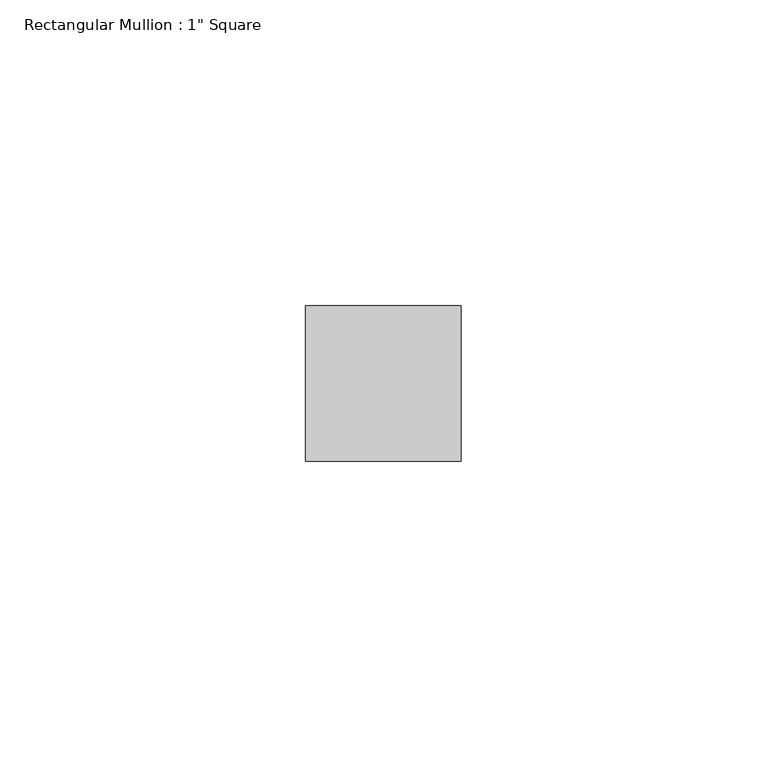
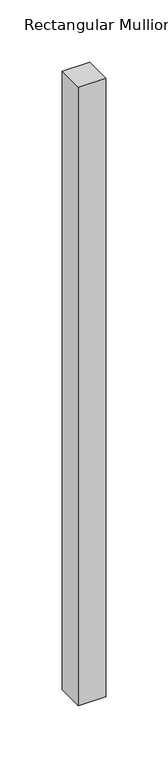
"""IFC4 building model written with IfcOpenShell, lengths in millimetres: member geometry."""

from ifc_helpers import new_model, si_unit, frame, origin, place, context, project, spatial, polyline, outline, extrude, source, transform, mapped, element, save


def member_cc9ef0d5(model_context):
    return source(origin(), model_context, "Body", "SweptSolid", [
        extrude(outline(polyline([(0.0, 12.7), (0.0, -12.7), (-25.4, -12.7), (-25.4, 12.7), (0.0, 12.7)])), frame((0.0, 0.0, -605.3666667), z_axis=(0.0, 0.0, 1.0), x_axis=(1.0, 0.0, 0.0)), (0.0, 0.0, 1.0), 605.3666667),
    ])


if __name__ == "__main__":
    model = new_model("IFC4")
    model_context = context("Model", 3, world=origin())
    ifc_project = project(units=[si_unit("LENGTHUNIT", "METRE", prefix="MILLI")], contexts=[model_context])
    site = spatial("IfcSite", under=ifc_project)
    building = spatial("IfcBuilding", under=site)
    placement = place(None, origin())
    member_shape = member_cc9ef0d5(model_context)
    element("IfcMember", 1, ObjectType="Rectangular Mullion : 1\" Square", at=placement, inside=building, context=model_context, shape_type="MappedRepresentation", body=[
        mapped(member_shape, transform((0.0, 0.0, 0.0), x_axis=(1.0, 0.0, 0.0), y_axis=(0.0, 1.0, 0.0), z_axis=(0.0, 0.0, 1.0))),
    ])
    save(model, "model.ifc")

# Revit data of these elements
# Type "Rectangular Mullion : 1\" Square"
#   built-in parameter 1007304 = 0.0833333 (stored number, unit not read)
#   built-in parameter 1007301 = 0.0416667 (stored number, unit not read)
#   built-in parameter 1007300 = 0.0416667 (stored number, unit not read)
# Element 1 (IfcMember, "Rectangular Mullion : 1\" Square")
#   Materials on its faces: "Aluminum"
# Materials
#   "Aluminum": class "Metal", colour RGB 247 247 247, transparency 0, Description = "Aluminum 6061", Cost = 0
